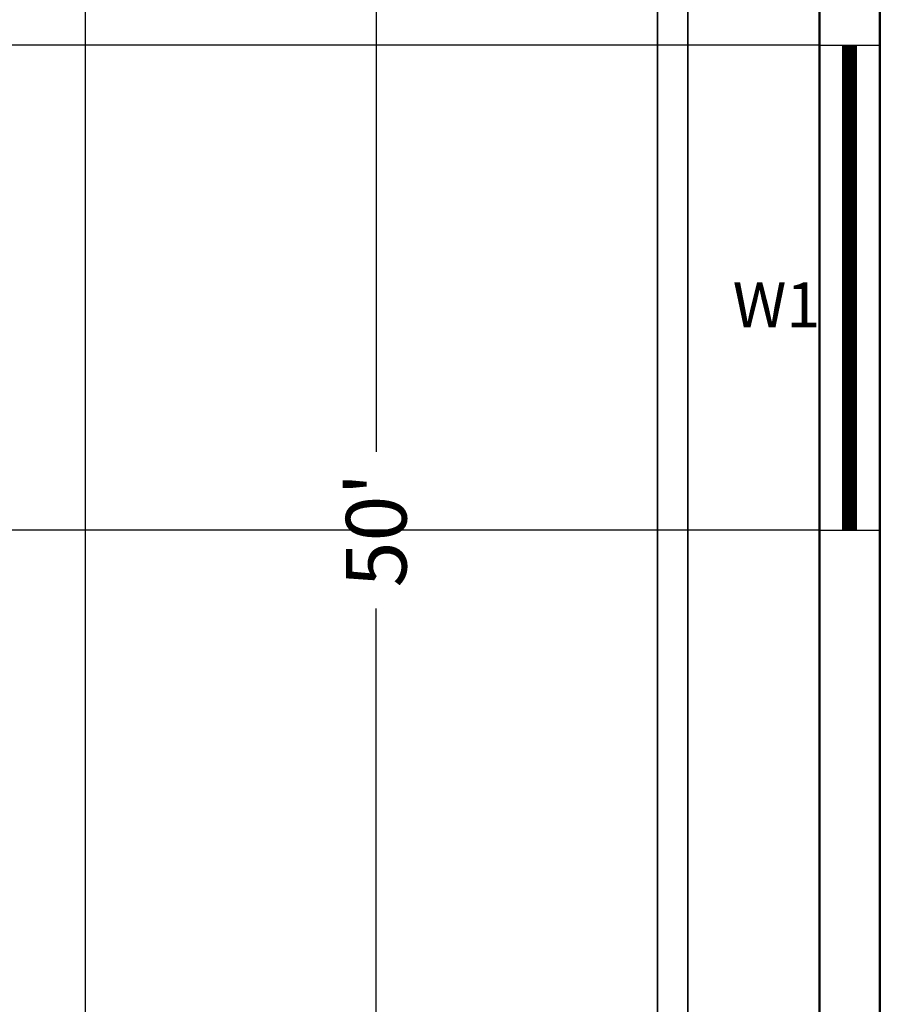
# Model space of a CAD drawing. Units: inches. Extents: x 338 to 1188, y -996 to 127.
# Tile 4 of 15: x 478 to 608, y -386 to -240. Entities that reach past the tile are written whole.
import ezdxf

# ---------------------------------------------------------------- set-up
doc = ezdxf.new("R2010")
doc.units = ezdxf.units.IN
doc.header["$MEASUREMENT"] = 0
for name, color, linetype, lineweight in [('A-ANNO-DIMS', 5, 'Continuous', 18), ('A-ANNO-TEXT', 7, 'Continuous', 18), ('A-GLAZ-PATT', 5, 'Continuous', 13), ('C-PROP', 1, 'Continuous', 35), ('wall', 1, 'Continuous', 50), ('win', 5, 'Continuous', 25)]:
    doc.layers.add(name, color=color, linetype=linetype, lineweight=lineweight)
doc.styles.get("Standard").update_dxf_attribs({"font": 'arial.ttf'})
doc.dimstyles.get("Standard").update_dxf_attribs({"dimtxt": 0.18, "dimasz": 0.18, "dimexe": 0.18, "dimexo": 0.0625, "dimgap": 0.09, "dimtad": 0, "dimtih": 1, "dimtoh": 1, "dimdec": 1, "dimzin": 0, "dimdsep": 46, "dimlunit": 4, "dimtxsty": 'Standard', "dimcen": 0.09, "dimadec": 0, "dimazin": 0, "dimtfac": 1, "dimtdec": 1, "dimtofl": 0, "dimtmove": 0, "dimatfit": 3, "dimfxl": 1, "dimtolj": 1, "dimtzin": 0, "dimarcsym": 0})

# ---------------------------------------------------------------- blocks, each defined once
blk = doc.blocks.new('_ArchTick')
at = {"color": 0, "linetype": 'ByBlock', "const_width": 0.15}
blk.add_lwpolyline([(-0.5, -0.5), (0.5, 0.5)], dxfattribs=at)
blk = doc.blocks.new('*D6')
at = {"layer": 'A-ANNO-DIMS', "color": 0, "lineweight": -2, "transparency": 16777216}
for p, q in [((531.19, -15.73), (531.19, -304.1)), ((531.19, -615.73), (531.19, -327.37))]:
    blk.add_line(p, q, dxfattribs=at)
at = {"layer": 'Defpoints', "color": 0, "transparency": 16777216}
for p in [(596.96, -15.73), (531.19, -615.73), (596.96, -615.73)]:
    blk.add_point(p, dxfattribs=at)
at = {"layer": 'A-ANNO-DIMS', "color": 0, "lineweight": -2, "transparency": 16777216, "xscale": 10, "yscale": 10, "zscale": 10}
for p, rotation in [((531.19, -15.73), 90), ((531.19, -615.73), 270)]:
    blk.add_blockref('_ArchTick', p, dxfattribs=dict(at, rotation=rotation))
at = {"layer": 'A-ANNO-DIMS', "color": 0, "transparency": 16777216, "insert": (531.19, -315.73), "char_height": 9, "attachment_point": 5, "rotation": 90}
blk.add_mtext("\\A1;50'", dxfattribs=at)
blk = doc.blocks.new('*D7')
at = {"layer": 'A-ANNO-DIMS', "color": 0, "lineweight": -2, "transparency": 16777216}
for p, q in [((488.01, 8.27), (488.01, -388.07)), ((488.01, -807.73), (488.01, -411.39))]:
    blk.add_line(p, q, dxfattribs=at)
at = {"layer": 'Defpoints', "color": 0, "transparency": 16777216}
for p in [(572.96, 8.27), (488.01, -807.73), (572.96, -807.73)]:
    blk.add_point(p, dxfattribs=at)
at = {"layer": 'A-ANNO-DIMS', "color": 0, "lineweight": -2, "transparency": 16777216, "xscale": 10, "yscale": 10, "zscale": 10}
for p, rotation in [((488.01, 8.27), 90), ((488.01, -807.73), 270)]:
    blk.add_blockref('_ArchTick', p, dxfattribs=dict(at, rotation=rotation))
at = {"layer": 'A-ANNO-DIMS', "color": 0, "transparency": 16777216, "insert": (488.01, -399.73), "char_height": 9, "attachment_point": 5, "rotation": 90}
blk.add_mtext("\\A1;68'", dxfattribs=at)
blk = doc.blocks.new('*D40')
at = {"layer": 'A-ANNO-DIMS', "color": 0, "lineweight": -2, "transparency": 16777216}
for p, q in [((596.9, -243.73), (337.66, -243.73)), ((337.84, -243.91), (337.84, -279.55)), ((337.84, -315.55), (337.84, -279.91)), ((596.9, -315.73), (337.66, -315.73))]:
    blk.add_line(p, q, dxfattribs=at)
at = {"layer": 'A-ANNO-DIMS', "color": 0, "transparency": 16777216}
for points in [[(337.81, -243.91), (337.87, -243.91), (337.84, -243.73)], [(337.81, -315.55), (337.87, -315.55), (337.84, -315.73)]]:
    blk.add_solid(points, dxfattribs=at)
at = {"layer": 'Defpoints', "color": 0, "transparency": 16777216}
for p in [(596.96, -243.73), (337.84, -315.73), (596.96, -315.73)]:
    blk.add_point(p, dxfattribs=at)
at = {"layer": 'A-ANNO-DIMS', "color": 0, "transparency": 16777216, "insert": (337.84, -279.73), "char_height": 0.18, "attachment_point": 5}
blk.add_mtext('\\A1;6\'-0"', dxfattribs=at)
blk = doc.blocks.new('*D48')
at = {"layer": 'A-ANNO-DIMS', "color": 0, "lineweight": -2, "transparency": 16777216}
for p, q in [((596.96, -615.67), (596.96, 67.25)), ((597.14, 67.07), (604.64, 67.07)), ((612.78, 67.07), (605.28, 67.07)), ((612.96, -615.67), (612.96, 67.25))]:
    blk.add_line(p, q, dxfattribs=at)
at = {"layer": 'A-ANNO-DIMS', "color": 0, "transparency": 16777216}
for points in [[(597.14, 67.1), (597.14, 67.04), (596.96, 67.07)], [(612.78, 67.1), (612.78, 67.04), (612.96, 67.07)]]:
    blk.add_solid(points, dxfattribs=at)
at = {"layer": 'Defpoints', "color": 0, "transparency": 16777216}
for p in [(612.96, 67.07), (596.96, -615.73), (612.96, -615.73)]:
    blk.add_point(p, dxfattribs=at)
at = {"layer": 'A-ANNO-DIMS', "color": 0, "transparency": 16777216, "insert": (604.96, 67.07), "char_height": 0.18, "attachment_point": 5}
blk.add_mtext('\\A1;1\'-4"', dxfattribs=at)
blk = doc.blocks.new('*D51')
at = {"layer": 'A-ANNO-DIMS', "color": 0, "lineweight": -2, "transparency": 16777216}
for p, q in [((596.9, -130.89), (337.66, -130.89)), ((337.84, -131.07), (337.84, -187.13)), ((337.84, -243.55), (337.84, -187.49)), ((596.9, -243.73), (337.66, -243.73))]:
    blk.add_line(p, q, dxfattribs=at)
at = {"layer": 'A-ANNO-DIMS', "color": 0, "transparency": 16777216}
for points in [[(337.81, -131.07), (337.87, -131.07), (337.84, -130.89)], [(337.81, -243.55), (337.87, -243.55), (337.84, -243.73)]]:
    blk.add_solid(points, dxfattribs=at)
at = {"layer": 'Defpoints', "color": 0, "transparency": 16777216}
for p in [(596.96, -130.89), (337.84, -243.73), (596.96, -243.73)]:
    blk.add_point(p, dxfattribs=at)
at = {"layer": 'A-ANNO-DIMS', "color": 0, "transparency": 16777216, "insert": (337.84, -187.31), "char_height": 0.18, "attachment_point": 5}
blk.add_mtext('\\A1;9\'-5"', dxfattribs=at)

msp = doc.modelspace()

# ---------------------------------------------------------------- hatches: boundary and pattern name
at = {"layer": 'A-GLAZ-PATT'}
h = msp.add_hatch(dxfattribs=at)
h.set_pattern_fill('ANSI31', color=256)
h.paths.add_polyline_path([(953.46, -405.07), (951.46, -405.07), (951.46, -429.07), (953.46, -429.07)])
h.paths.add_polyline_path([(953.46, -485.22), (951.46, -485.22), (951.46, -521.22), (953.46, -521.22)])
h.paths.add_polyline_path([(794.21, -19.23), (758.21, -19.23), (758.21, -21.23), (794.21, -21.23)])
h.paths.add_polyline_path([(668.69, -19.23), (632.69, -19.23), (632.69, -21.23), (668.69, -21.23)])
h.paths.add_polyline_path([(602.46, -94.89), (600.46, -94.89), (600.46, -130.89), (602.46, -130.89)])
h.paths.add_polyline_path([(602.46, -243.73), (600.46, -243.73), (600.46, -315.73), (602.46, -315.73)])

# ---------------------------------------------------------------- linework, layer by layer
at = {"layer": 'C-PROP'}
for p, q in [((572.96, 8.27), (572.96, -807.73)), ((577.46, 3.77), (577.46, -803.23))]:
    msp.add_line(p, q, dxfattribs=at)
at = {"layer": 'wall'}
for p, q in [((596.96, -15.73), (596.96, -615.73)), ((605.96, -149.23), (605.96, -606.73))]:
    msp.add_line(p, q, dxfattribs=at)
at = {"layer": 'win'}
for p, q in [((596.96, -243.73), (605.96, -243.73)), ((600.46, -315.73), (600.46, -243.73)), ((602.46, -315.73), (602.46, -243.73)), ((596.96, -315.73), (605.96, -315.73))]:
    msp.add_line(p, q, dxfattribs=at)

# ---------------------------------------------------------------- texts
at = {"layer": 'A-ANNO-TEXT'}
msp.add_text('W1', height=6.652, dxfattribs=at).set_placement((584.1, -285.62))

# ---------------------------------------------------------------- dimensions: what is measured, and where the dimension line sits
at = {"layer": 'A-ANNO-DIMS'}
dim = msp.add_linear_dim(base=(612.96, 67.07), p1=(596.96, -615.73), p2=(612.96, -615.73), dimstyle='Standard', override={"dimdec": 1, "dimlfac": 1, "dimrnd": 0, "dimzin": 1, "dimdsep": 46, "dimlunit": 4, "dimfrac": 2}, dxfattribs=at)
dim.commit()
dim.dimension.update_dxf_attribs({"geometry": '*D48', "text_midpoint": (604.96, 67.07)})
for base, p1, p2, override, picture, middle in [((488.01, -807.73), (572.96, 8.27), (572.96, -807.73), {"dimtxt": 9, "dimasz": 10, "dimgap": 4, "dimtad": 0, "dimtih": 0, "dimblk1": 'ArchTick', "dimblk2": 'ArchTick', "dimsah": 1, "dimse1": 1, "dimse2": 1, "dimclrd": 0, "dimclre": 0, "dimclrt": 0}, '*D7', (488.01, -399.73)), ((531.19, -615.73), (596.96, -15.73), (596.96, -615.73), {"dimtxt": 9, "dimasz": 10, "dimgap": 4, "dimtih": 0, "dimblk1": 'ArchTick', "dimblk2": 'ArchTick', "dimsah": 1, "dimse1": 1, "dimse2": 1, "dimclrd": 0, "dimclre": 0, "dimclrt": 0}, '*D6', (531.19, -315.73)), ((337.84, -243.73), (596.96, -130.89), (596.96, -243.73), {"dimdec": 1, "dimlfac": 1, "dimrnd": 0, "dimzin": 1, "dimdsep": 46, "dimlunit": 4, "dimfrac": 2}, '*D51', (337.84, -187.31)), ((337.84, -315.73), (596.96, -243.73), (596.96, -315.73), {"dimdec": 1, "dimlfac": 1, "dimrnd": 0, "dimzin": 1, "dimdsep": 46, "dimlunit": 4, "dimfrac": 2}, '*D40', (337.84, -279.73))]:
    dim = msp.add_linear_dim(base=base, p1=p1, p2=p2, angle=90, dimstyle='Standard', override=override, dxfattribs=at)
    dim.commit()
    dim.dimension.update_dxf_attribs({"geometry": picture, "text_midpoint": middle})

doc.saveas('drawing.dxf')
